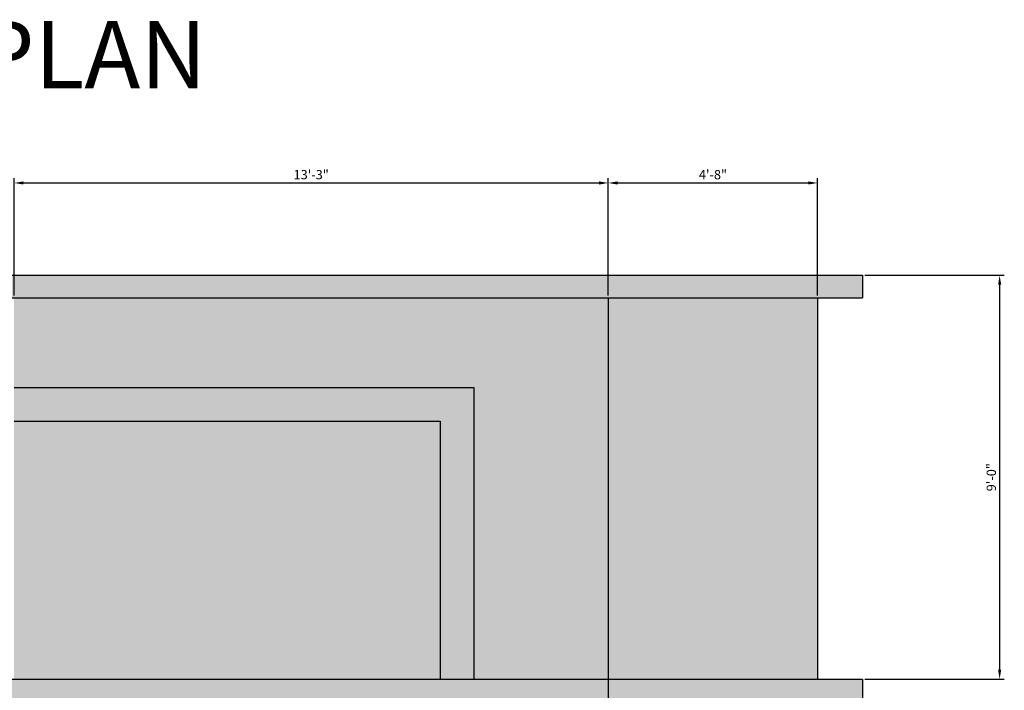
# Model space of a CAD drawing. Units: inches. Extents: x 2169 to 10664, y 1669 to 6352.
# Tile 15 of 17: x 9778 to 10041, y 5441 to 5621. Entities that reach past the tile are written whole.
import ezdxf

# ---------------------------------------------------------------- set-up
doc = ezdxf.new("R2010")
doc.units = ezdxf.units.IN
for name, color, linetype, lineweight in [('A-ANNO-DIMS', 3, 'Continuous', 18), ('A-ANNO-TITL', 3, 'Continuous', 25), ('A-ELEV', 7, 'Continuous', 25), ('A-ELEV-CONC-PATT', 85, 'Continuous', 13), ('A-ELEV-PATT', 253, 'Continuous', 13)]:
    doc.layers.add(name, color=color, linetype=linetype, lineweight=lineweight)
doc.styles.get("Standard").update_dxf_attribs({"font": 'arial.ttf'})
doc.dimstyles.new('ISO-25', dxfattribs={"dimtxt": 2.5, "dimasz": 2.5, "dimexe": 1.25, "dimexo": 0.625, "dimtad": 1, "dimdec": 0, "dimlunit": 3, "dimtxsty": 'Standard', "dimcen": 2.5, "dimadec": 0, "dimazin": 0, "dimtfac": 1, "dimtdec": 0, "dimtmove": 0, "dimatfit": 3, "dimfxl": 1, "dimarcsym": 0})

# ---------------------------------------------------------------- blocks, each defined once
blk = doc.blocks.new('*D119')
at = {"layer": 'A-ANNO-DIMS', "color": 0, "lineweight": -2, "transparency": 16777216}
for p, q in [((10004.09, 5552.31), (10041.41, 5552.31)), ((10040.16, 5549.81), (10040.16, 5446.81)), ((10004.09, 5444.31), (10041.41, 5444.31))]:
    blk.add_line(p, q, dxfattribs=at)
at = {"layer": 'A-ANNO-DIMS', "color": 0, "transparency": 16777216}
for points in [[(10039.75, 5549.81), (10040.58, 5549.81), (10040.16, 5552.31)], [(10039.75, 5446.81), (10040.58, 5446.81), (10040.16, 5444.31)]]:
    blk.add_solid(points, dxfattribs=at)
at = {"layer": 'Defpoints', "color": 0, "transparency": 16777216}
for p in [(10003.46, 5552.31), (10003.46, 5444.31), (10040.16, 5444.31)]:
    blk.add_point(p, dxfattribs=at)
at = {"layer": 'A-ANNO-DIMS', "color": 0, "transparency": 16777216, "insert": (10038.26, 5498.31), "char_height": 2.5, "attachment_point": 5, "rotation": 90}
blk.add_mtext('9\'-0"', dxfattribs=at)
blk = doc.blocks.new('*D122')
at = {"layer": 'A-ANNO-DIMS', "color": 0, "lineweight": -2, "transparency": 16777216}
for p, q in [((9776.46, 5546.94), (9776.46, 5578.26)), ((9935.46, 5546.94), (9935.46, 5578.26)), ((9778.96, 5577.01), (9932.96, 5577.01))]:
    blk.add_line(p, q, dxfattribs=at)
at = {"layer": 'A-ANNO-DIMS', "color": 0, "transparency": 16777216}
for points in [[(9778.96, 5577.43), (9778.96, 5576.59), (9776.46, 5577.01)], [(9932.96, 5577.43), (9932.96, 5576.59), (9935.46, 5577.01)]]:
    blk.add_solid(points, dxfattribs=at)
at = {"layer": 'Defpoints', "color": 0, "transparency": 16777216}
for p in [(9935.46, 5577.01), (9776.46, 5546.31), (9935.46, 5546.31)]:
    blk.add_point(p, dxfattribs=at)
at = {"layer": 'A-ANNO-DIMS', "color": 0, "transparency": 16777216, "insert": (9855.96, 5578.91), "char_height": 2.5, "attachment_point": 5}
blk.add_mtext('13\'-3"', dxfattribs=at)
blk = doc.blocks.new('*D123')
at = {"layer": 'A-ANNO-DIMS', "color": 0, "lineweight": -2, "transparency": 16777216}
for p, q in [((9935.46, 5546.94), (9935.46, 5578.26)), ((9991.46, 5546.94), (9991.46, 5578.26)), ((9937.96, 5577.01), (9988.96, 5577.01))]:
    blk.add_line(p, q, dxfattribs=at)
at = {"layer": 'A-ANNO-DIMS', "color": 0, "transparency": 16777216}
for points in [[(9937.96, 5577.43), (9937.96, 5576.59), (9935.46, 5577.01)], [(9988.96, 5577.43), (9988.96, 5576.59), (9991.46, 5577.01)]]:
    blk.add_solid(points, dxfattribs=at)
at = {"layer": 'Defpoints', "color": 0, "transparency": 16777216}
for p in [(9991.46, 5577.01), (9935.46, 5546.31), (9991.46, 5546.31)]:
    blk.add_point(p, dxfattribs=at)
at = {"layer": 'A-ANNO-DIMS', "color": 0, "transparency": 16777216, "insert": (9963.46, 5578.91), "char_height": 2.5, "attachment_point": 5}
blk.add_mtext('4\'-8"', dxfattribs=at)

msp = doc.modelspace()

# ---------------------------------------------------------------- hatches: boundary and pattern name
at = {"layer": 'A-ELEV-CONC-PATT'}
h = msp.add_hatch(dxfattribs=at)
h.set_pattern_fill('AR-CONC', color=256, scale=0.02)
h.paths.add_polyline_path([(9899.46, 5522.31), (9776.46, 5522.31), (9776.46, 5513.31), (9890.46, 5513.31), (9890.46, 5444.31), (9899.46, 5444.31)])
h.paths.add_polyline_path([(9899.46, 5438.31), (9890.46, 5438.31), (9890.46, 5285.31), (9899.46, 5285.31)])
at = {"layer": 'A-ELEV-PATT'}
h = msp.add_hatch(color=256, dxfattribs=at)
h.dxf.hatch_style = 1
h.paths.add_polyline_path([(10003.46, 5552.31), (9547.46, 5552.31), (9547.46, 5546.31), (10003.46, 5546.31)])
h.paths.add_polyline_path([(9776.46, 5444.31), (9547.46, 5444.31), (9547.46, 5438.31), (9776.46, 5438.31)])
h.paths.add_polyline_path([(9935.46, 5444.31), (9776.46, 5444.31), (9776.46, 5438.31), (9935.46, 5438.31)])
h.paths.add_polyline_path([(10003.46, 5444.31), (9935.46, 5444.31), (9935.46, 5438.31), (10003.46, 5438.31)])
h = msp.add_hatch(color=256, dxfattribs=at)
h.dxf.hatch_style = 1
h.paths.add_polyline_path([(9935.46, 5546.31), (9776.46, 5546.31), (9776.46, 5522.31), (9899.46, 5522.31), (9899.46, 5444.31), (9935.46, 5444.31)])
h.paths.add_polyline_path([(9935.46, 5438.31), (9899.46, 5438.31), (9899.46, 5285.31), (9935.46, 5285.31)])
h.paths.add_polyline_path([(9890.46, 5438.31), (9848.46, 5438.31), (9848.46, 5285.31), (9890.46, 5285.31)])
h.paths.add_polyline_path([(9890.46, 5513.31), (9776.46, 5513.31), (9776.46, 5444.31), (9890.46, 5444.31)], flags=17)
h = msp.add_hatch(color=256, dxfattribs=at)
h.dxf.hatch_style = 1
h.paths.add_polyline_path([(9991.46, 5438.31), (9935.46, 5438.31), (9935.46, 5360.31), (9991.46, 5360.31)])
h.paths.add_polyline_path([(9991.46, 5546.31), (9935.46, 5546.31), (9935.46, 5444.31), (9991.46, 5444.31)])

# ---------------------------------------------------------------- linework, layer by layer
at = {"layer": 'A-ELEV'}
for p, q in [((9547.46, 5552.31), (10003.46, 5552.31)), ((10003.46, 5552.31), (10003.46, 5546.31)), ((9547.46, 5546.31), (10003.46, 5546.31)), ((9935.46, 5546.31), (9935.46, 5285.31)), ((9991.46, 5546.31), (9991.46, 5444.31)), ((9776.46, 5522.31), (9899.46, 5522.31)), ((9899.46, 5522.31), (9899.46, 5444.31)), ((9776.46, 5513.31), (9890.46, 5513.31)), ((9890.46, 5513.31), (9890.46, 5444.31)), ((9547.46, 5444.31), (9935.46, 5444.31)), ((9935.46, 5444.31), (10003.46, 5444.31)), ((10003.46, 5444.31), (10003.46, 5438.31))]:
    msp.add_line(p, q, dxfattribs=at)

# ---------------------------------------------------------------- texts
at = {"layer": 'A-ANNO-TITL', "insert": (9681.98, 5620.36), "char_height": 18, "attachment_point": 1}
msp.add_mtext_dynamic_manual_height_columns('FLOOR PLAN', width=475.2595, gutter_width=12.5, heights=[0], dxfattribs=at)

# ---------------------------------------------------------------- dimensions: what is measured, and where the dimension line sits
at = {"layer": 'A-ANNO-DIMS'}
for base, p1, p2, picture, middle in [((9935.46, 5577.01), (9776.46, 5546.31), (9935.46, 5546.31), '*D122', (9855.96, 5578.91)), ((9991.46, 5577.01), (9935.46, 5546.31), (9991.46, 5546.31), '*D123', (9963.46, 5578.91))]:
    dim = msp.add_linear_dim(base=base, p1=p1, p2=p2, dimstyle='ISO-25', override={"dimdec": 1, "dimlfac": 1, "dimrnd": 0, "dimzin": 1, "dimdsep": 46, "dimlunit": 4, "dimfrac": 2}, dxfattribs=at)
    dim.commit()
    dim.dimension.update_dxf_attribs({"geometry": picture, "text_midpoint": middle})
dim = msp.add_linear_dim(base=(10040.16, 5444.31), p1=(10003.46, 5552.31), p2=(10003.46, 5444.31), angle=90, dimstyle='ISO-25', override={"dimdec": 1, "dimlfac": 1, "dimrnd": 0, "dimzin": 1, "dimdsep": 46, "dimlunit": 4, "dimfrac": 2}, dxfattribs=at)
dim.commit()
dim.dimension.update_dxf_attribs({"geometry": '*D119', "text_midpoint": (10038.26, 5498.31)})

doc.saveas('drawing.dxf')
